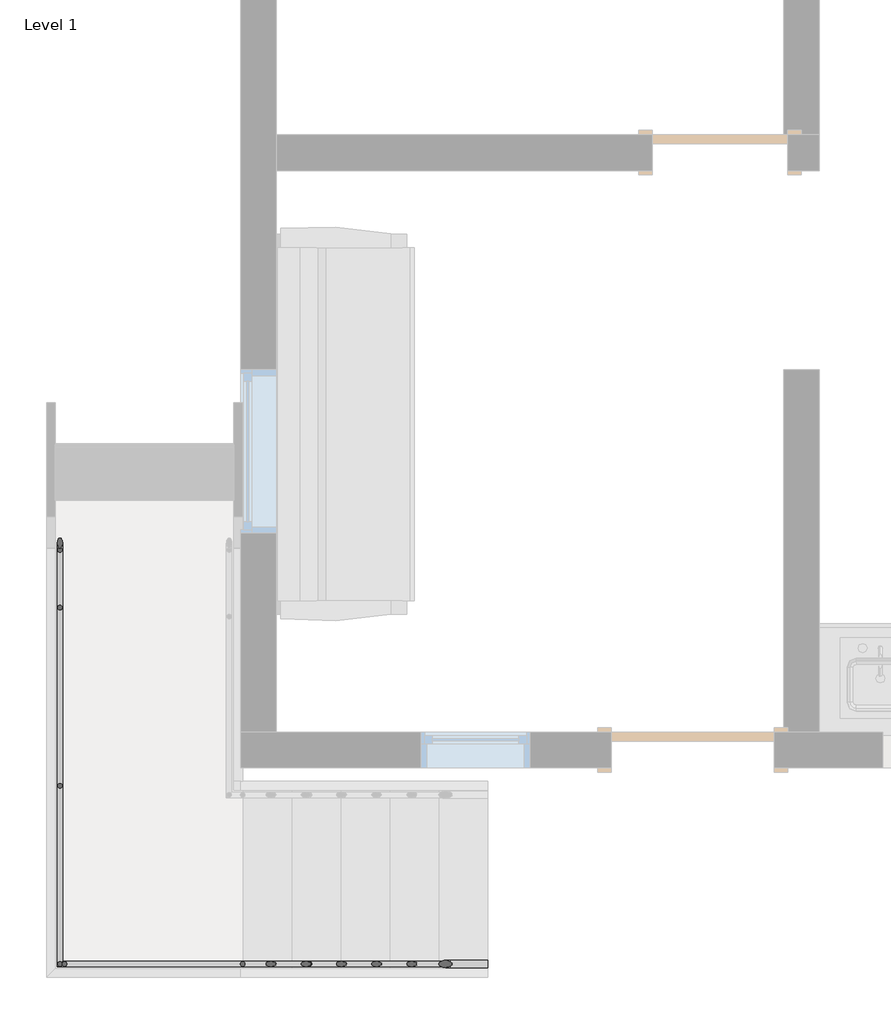
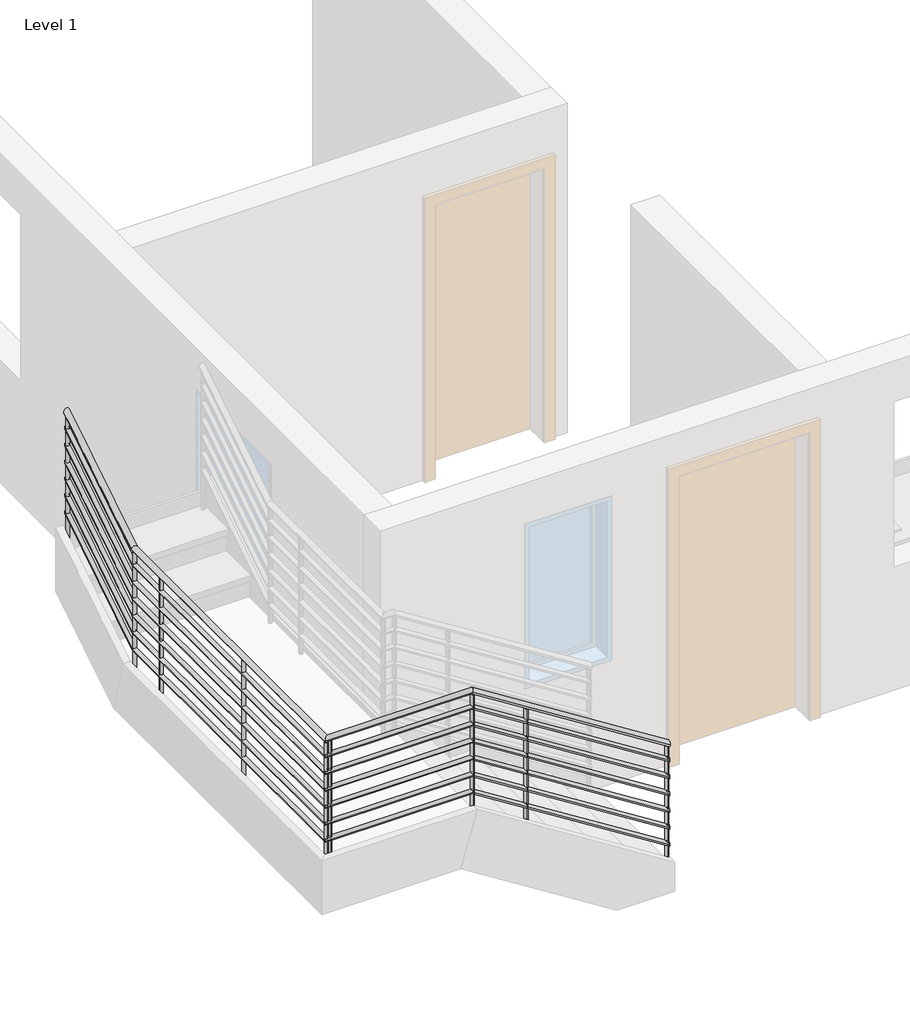
# One storey, part 2 of 3: 1 railing.
"""IFC4 building model written with IfcOpenShell, lengths in millimetres."""

from ifc_helpers import new_model, si_unit, point, frame, frame_2d, origin, place, context, project, spatial, circle_curve, ellipse_curve, trimmed, segment, composite_curve, outline, extrude, element, save
from ifc_brep_helpers import plane_surface, cylinder_surface, advanced_brep

model = new_model("IFC4")

# Units and contexts
model_context = context("Model", 3, world=origin())
ifc_project = project(units=[si_unit("LENGTHUNIT", "METRE", prefix="MILLI")], contexts=[model_context])

# Site, building, storey
site = spatial("IfcSite", under=ifc_project)
building = spatial("IfcBuilding", under=site)
storey = spatial("IfcBuildingStorey", under=building, Name="Level 1", Elevation=0.0)

# Railing
placement = place(None, origin())
element("IfcRailing", 1, ObjectType="900mm Pipe", at=placement, inside=storey, context=model_context, shape_type="SolidModel", body=[
    advanced_brep(
    [(-10176.2529994, 4755.2403022, 1050.2491997), (-10176.2529994, 4715.2403022, 1050.2491997), (-11557.0464524, 4755.2403022, 1923.4782609), (-11557.0464524, 4715.2403022, 1923.4782609), (-12556.6787807, 4755.2403022, 1923.4782609), (-12596.6787807, 4715.2403022, 1923.4782609), (-12556.6787807, 7064.6595365, 1923.4782609), (-12596.6787807, 7064.6595365, 1923.4782609), (-12556.6787807, 7883.8660835, 2441.5535475), (-12596.6787807, 7883.8660835, 2441.5535475)],
    [
        (0, 1, ellipse_curve(frame((-10176.2529994, 4735.2403022, 1050.2491997), z_axis=(1.0, 0.0, 0.0), x_axis=(0.0, 0.0, -1.0)), 23.6638438, 20.0)),
        (1, 0, ellipse_curve(frame((-10176.2529994, 4735.2403022, 1050.2491997), z_axis=(1.0, 0.0, 0.0), x_axis=(0.0, 0.0, -1.0)), 23.6638438, 20.0)),
        (0, 2),
        (2, 3, ellipse_curve(frame((-11557.0464524, 4735.2403022, 1923.4782609), z_axis=(0.9605132043335073, 0.0, -0.2782344053149754), x_axis=(-0.278234405314975, 0.0, -0.9605132043335074)), 20.822202, 20.0)),
        (3, 1),
        (3, 2, ellipse_curve(frame((-11557.0464524, 4735.2403022, 1923.4782609), z_axis=(0.9605132043335073, 0.0, -0.2782344053149754), x_axis=(-0.278234405314975, 0.0, -0.9605132043335074)), 20.822202, 20.0)),
        (2, 4),
        (4, 5, ellipse_curve(frame((-12576.6787807, 4735.2403022, 1923.4782609), z_axis=(0.7071067811865425, -0.7071067811865526, 0.0), x_axis=(0.7071067811865526, 0.7071067811865424, 0.0)), 28.2842712, 20.0)),
        (5, 3),
        (5, 4, ellipse_curve(frame((-12576.6787807, 4735.2403022, 1923.4782609), z_axis=(0.7071067811865425, -0.7071067811865526, 0.0), x_axis=(0.7071067811865526, 0.7071067811865424, 0.0)), 28.2842712, 20.0)),
        (4, 6),
        (6, 7, ellipse_curve(frame((-12576.6787807, 7064.6595365, 1923.4782609), z_axis=(0.0, -0.9605132043335083, -0.27823440531497184), x_axis=(0.0, -0.27823440531497223, 0.9605132043335083)), 20.822202, 20.0)),
        (7, 5),
        (7, 6, ellipse_curve(frame((-12576.6787807, 7064.6595365, 1923.4782609), z_axis=(0.0, -0.9605132043335083, -0.27823440531497184), x_axis=(0.0, -0.27823440531497223, 0.9605132043335083)), 20.822202, 20.0)),
        (8, 9, ellipse_curve(frame((-12576.6787807, 7883.8660835, 2441.5535475), z_axis=(0.0, 1.0, 0.0), x_axis=(0.0, 0.0, -1.0)), 23.6638438, 20.0)),
        (9, 8, ellipse_curve(frame((-12576.6787807, 7883.8660835, 2441.5535475), z_axis=(0.0, 1.0, 0.0), x_axis=(0.0, 0.0, -1.0)), 23.6638438, 20.0)),
        (6, 8),
        (9, 7),
    ],
    [
        plane_surface(frame((-10176.2529994, 4735.2403022, 1073.9130435), z_axis=(1.0, 0.0, 0.0), x_axis=(0.0, -1.0, 0.0))),
        cylinder_surface(frame((-10186.9429122, 4735.2403022, 1057.0096189), z_axis=(0.845171231398044, 0.0, -0.5344956404098298), x_axis=(0.0, -1.0, 0.0)), 20.0),
        cylinder_surface(frame((-11551.2529994, 4735.2403022, 1923.4782609), z_axis=(1.0, 0.0, 0.0), x_axis=(0.0, -1.0, 0.0)), 20.0),
        cylinder_surface(frame((-12576.6787807, 4735.2403022, 1923.4782609), z_axis=(0.0, -1.0, 0.0), x_axis=(-1.0, 0.0, 0.0)), 20.0),
        plane_surface(frame((-12576.6787807, 7883.8660835, 2465.2173913), z_axis=(0.0, 1.0, 0.0), x_axis=(0.0, 0.0, 1.0))),
        cylinder_surface(frame((-12576.6787807, 7069.5559963, 1926.5748362), z_axis=(0.0, -0.845171231398048, -0.5344956404098234), x_axis=(-1.0, 0.0, 0.0)), 20.0),
    ],
    [
        (0, [[1, 2]]),
        (1, [[-1, 3, 4, 5]]),
        (1, [[-2, -5, 6, -3]]),
        (2, [[-4, 7, 8, 9]]),
        (2, [[-6, -9, 10, -7]]),
        (3, [[-8, 11, 12, 13]]),
        (3, [[-10, -13, 14, -11]]),
        (4, [[15, 16]]),
        (5, [[-12, 17, -16, 18]]),
        (5, [[-14, -18, -15, -17]]),
    ],
),
    advanced_brep(
    [(-10176.2529994, 4750.2403022, 931.1651606), (-10176.2529994, 4720.2403022, 931.1651606), (-11555.5980892, 4750.2403022, 1803.4782609), (-11555.5980892, 4720.2403022, 1803.4782609), (-12561.6787807, 4750.2403022, 1803.4782609), (-12591.6787807, 4720.2403022, 1803.4782609), (-12561.6787807, 7063.2111733, 1803.4782609), (-12591.6787807, 7063.2111733, 1803.4782609), (-12561.6787807, 7883.8660835, 2322.4695085), (-12591.6787807, 7883.8660835, 2322.4695085)],
    [
        (0, 1, ellipse_curve(frame((-10176.2529994, 4735.2403022, 931.1651606), z_axis=(1.0, 0.0, 0.0), x_axis=(0.0, 0.0, -1.0)), 17.7478828, 15.0)),
        (1, 0, ellipse_curve(frame((-10176.2529994, 4735.2403022, 931.1651606), z_axis=(1.0, 0.0, 0.0), x_axis=(0.0, 0.0, -1.0)), 17.7478828, 15.0)),
        (0, 2),
        (2, 3, ellipse_curve(frame((-11555.5980892, 4735.2403022, 1803.4782609), z_axis=(0.9605132043335073, 0.0, -0.27823440531497534), x_axis=(-0.27823440531497506, 0.0, -0.9605132043335075)), 15.6166515, 15.0)),
        (3, 1),
        (3, 2, ellipse_curve(frame((-11555.5980892, 4735.2403022, 1803.4782609), z_axis=(0.9605132043335073, 0.0, -0.27823440531497534), x_axis=(-0.27823440531497506, 0.0, -0.9605132043335075)), 15.6166515, 15.0)),
        (2, 4),
        (4, 5, ellipse_curve(frame((-12576.6787807, 4735.2403022, 1803.4782609), z_axis=(0.7071067811865425, -0.7071067811865526, 0.0), x_axis=(0.7071067811865526, 0.7071067811865424, 0.0)), 21.2132034, 15.0)),
        (5, 3),
        (5, 4, ellipse_curve(frame((-12576.6787807, 4735.2403022, 1803.4782609), z_axis=(0.7071067811865425, -0.7071067811865526, 0.0), x_axis=(0.7071067811865526, 0.7071067811865424, 0.0)), 21.2132034, 15.0)),
        (4, 6),
        (6, 7, ellipse_curve(frame((-12576.6787807, 7063.2111733, 1803.4782609), z_axis=(0.0, -0.9605132043335083, -0.27823440531497196), x_axis=(0.0, -0.2782344053149721, 0.9605132043335084)), 15.6166515, 15.0)),
        (7, 5),
        (7, 6, ellipse_curve(frame((-12576.6787807, 7063.2111733, 1803.4782609), z_axis=(0.0, -0.9605132043335083, -0.27823440531497196), x_axis=(0.0, -0.2782344053149721, 0.9605132043335084)), 15.6166515, 15.0)),
        (8, 9, ellipse_curve(frame((-12576.6787807, 7883.8660835, 2322.4695085), z_axis=(0.0, 1.0, 0.0), x_axis=(0.0, 0.0, -1.0)), 17.7478828, 15.0)),
        (9, 8, ellipse_curve(frame((-12576.6787807, 7883.8660835, 2322.4695085), z_axis=(0.0, 1.0, 0.0), x_axis=(0.0, 0.0, -1.0)), 17.7478828, 15.0)),
        (6, 8),
        (9, 7),
    ],
    [
        plane_surface(frame((-10176.2529994, 4735.2403022, 948.9130435), z_axis=(1.0, 0.0, 0.0), x_axis=(0.0, -1.0, 0.0))),
        cylinder_surface(frame((-10184.270434, 4735.2403022, 936.235475), z_axis=(0.845171231398044, 0.0, -0.5344956404098297), x_axis=(0.0, -1.0, 0.0)), 15.0),
        cylinder_surface(frame((-11551.2529994, 4735.2403022, 1803.4782609), z_axis=(1.0, 0.0, 0.0), x_axis=(0.0, -1.0, 0.0)), 15.0),
        cylinder_surface(frame((-12576.6787807, 4735.2403022, 1803.4782609), z_axis=(0.0, -1.0, 0.0), x_axis=(-1.0, 0.0, 0.0)), 15.0),
        plane_surface(frame((-12576.6787807, 7883.8660835, 2340.2173913), z_axis=(0.0, 1.0, 0.0), x_axis=(0.0, 0.0, 1.0))),
        cylinder_surface(frame((-12576.6787807, 7066.8835181, 1805.8006924), z_axis=(0.0, -0.8451712313980478, -0.5344956404098237), x_axis=(-1.0, 0.0, 0.0)), 15.0),
    ],
    [
        (0, [[1, 2]]),
        (1, [[-1, 3, 4, 5]]),
        (1, [[-2, -5, 6, -3]]),
        (2, [[-4, 7, 8, 9]]),
        (2, [[-6, -9, 10, -7]]),
        (3, [[-8, 11, 12, 13]]),
        (3, [[-10, -13, 14, -11]]),
        (4, [[15, 16]]),
        (5, [[-12, 17, -16, 18]]),
        (5, [[-14, -18, -15, -17]]),
    ],
),
    advanced_brep(
    [(-10176.2529994, 4750.2403022, 806.1651606), (-10176.2529994, 4720.2403022, 806.1651606), (-11555.5980892, 4750.2403022, 1678.4782609), (-11555.5980892, 4720.2403022, 1678.4782609), (-12561.6787807, 4750.2403022, 1678.4782609), (-12591.6787807, 4720.2403022, 1678.4782609), (-12561.6787807, 7063.2111733, 1678.4782609), (-12591.6787807, 7063.2111733, 1678.4782609), (-12561.6787807, 7883.8660835, 2197.4695085), (-12591.6787807, 7883.8660835, 2197.4695085)],
    [
        (0, 1, ellipse_curve(frame((-10176.2529994, 4735.2403022, 806.1651606), z_axis=(1.0, 0.0, 0.0), x_axis=(0.0, 0.0, -1.0)), 17.7478828, 15.0)),
        (1, 0, ellipse_curve(frame((-10176.2529994, 4735.2403022, 806.1651606), z_axis=(1.0, 0.0, 0.0), x_axis=(0.0, 0.0, -1.0)), 17.7478828, 15.0)),
        (0, 2),
        (2, 3, ellipse_curve(frame((-11555.5980892, 4735.2403022, 1678.4782609), z_axis=(0.9605132043335073, 0.0, -0.27823440531497534), x_axis=(-0.27823440531497506, 0.0, -0.9605132043335075)), 15.6166515, 15.0)),
        (3, 1),
        (3, 2, ellipse_curve(frame((-11555.5980892, 4735.2403022, 1678.4782609), z_axis=(0.9605132043335073, 0.0, -0.27823440531497534), x_axis=(-0.27823440531497506, 0.0, -0.9605132043335075)), 15.6166515, 15.0)),
        (2, 4),
        (4, 5, ellipse_curve(frame((-12576.6787807, 4735.2403022, 1678.4782609), z_axis=(0.7071067811865425, -0.7071067811865526, 0.0), x_axis=(0.7071067811865526, 0.7071067811865424, 0.0)), 21.2132034, 15.0)),
        (5, 3),
        (5, 4, ellipse_curve(frame((-12576.6787807, 4735.2403022, 1678.4782609), z_axis=(0.7071067811865425, -0.7071067811865526, 0.0), x_axis=(0.7071067811865526, 0.7071067811865424, 0.0)), 21.2132034, 15.0)),
        (4, 6),
        (6, 7, ellipse_curve(frame((-12576.6787807, 7063.2111733, 1678.4782609), z_axis=(0.0, -0.9605132043335083, -0.27823440531497196), x_axis=(0.0, -0.2782344053149721, 0.9605132043335084)), 15.6166515, 15.0)),
        (7, 5),
        (7, 6, ellipse_curve(frame((-12576.6787807, 7063.2111733, 1678.4782609), z_axis=(0.0, -0.9605132043335083, -0.27823440531497196), x_axis=(0.0, -0.2782344053149721, 0.9605132043335084)), 15.6166515, 15.0)),
        (8, 9, ellipse_curve(frame((-12576.6787807, 7883.8660835, 2197.4695085), z_axis=(0.0, 1.0, 0.0), x_axis=(0.0, 0.0, -1.0)), 17.7478828, 15.0)),
        (9, 8, ellipse_curve(frame((-12576.6787807, 7883.8660835, 2197.4695085), z_axis=(0.0, 1.0, 0.0), x_axis=(0.0, 0.0, -1.0)), 17.7478828, 15.0)),
        (6, 8),
        (9, 7),
    ],
    [
        plane_surface(frame((-10176.2529994, 4735.2403022, 823.9130435), z_axis=(1.0, 0.0, 0.0), x_axis=(0.0, -1.0, 0.0))),
        cylinder_surface(frame((-10184.270434, 4735.2403022, 811.235475), z_axis=(0.845171231398044, 0.0, -0.5344956404098297), x_axis=(0.0, -1.0, 0.0)), 15.0),
        cylinder_surface(frame((-11551.2529994, 4735.2403022, 1678.4782609), z_axis=(1.0, 0.0, 0.0), x_axis=(0.0, -1.0, 0.0)), 15.0),
        cylinder_surface(frame((-12576.6787807, 4735.2403022, 1678.4782609), z_axis=(0.0, -1.0, 0.0), x_axis=(-1.0, 0.0, 0.0)), 15.0),
        plane_surface(frame((-12576.6787807, 7883.8660835, 2215.2173913), z_axis=(0.0, 1.0, 0.0), x_axis=(0.0, 0.0, 1.0))),
        cylinder_surface(frame((-12576.6787807, 7066.8835181, 1680.8006924), z_axis=(0.0, -0.8451712313980478, -0.5344956404098237), x_axis=(-1.0, 0.0, 0.0)), 15.0),
    ],
    [
        (0, [[1, 2]]),
        (1, [[-1, 3, 4, 5]]),
        (1, [[-2, -5, 6, -3]]),
        (2, [[-4, 7, 8, 9]]),
        (2, [[-6, -9, 10, -7]]),
        (3, [[-8, 11, 12, 13]]),
        (3, [[-10, -13, 14, -11]]),
        (4, [[15, 16]]),
        (5, [[-12, 17, -16, 18]]),
        (5, [[-14, -18, -15, -17]]),
    ],
),
    advanced_brep(
    [(-10176.2529994, 4750.2403022, 681.1651606), (-10176.2529994, 4720.2403022, 681.1651606), (-11555.5980892, 4750.2403022, 1553.4782609), (-11555.5980892, 4720.2403022, 1553.4782609), (-12561.6787807, 4750.2403022, 1553.4782609), (-12591.6787807, 4720.2403022, 1553.4782609), (-12561.6787807, 7063.2111733, 1553.4782609), (-12591.6787807, 7063.2111733, 1553.4782609), (-12561.6787807, 7883.8660835, 2072.4695085), (-12591.6787807, 7883.8660835, 2072.4695085)],
    [
        (0, 1, ellipse_curve(frame((-10176.2529994, 4735.2403022, 681.1651606), z_axis=(1.0, 0.0, 0.0), x_axis=(0.0, 0.0, -1.0)), 17.7478828, 15.0)),
        (1, 0, ellipse_curve(frame((-10176.2529994, 4735.2403022, 681.1651606), z_axis=(1.0, 0.0, 0.0), x_axis=(0.0, 0.0, -1.0)), 17.7478828, 15.0)),
        (0, 2),
        (2, 3, ellipse_curve(frame((-11555.5980892, 4735.2403022, 1553.4782609), z_axis=(0.9605132043335073, 0.0, -0.27823440531497534), x_axis=(-0.27823440531497506, 0.0, -0.9605132043335075)), 15.6166515, 15.0)),
        (3, 1),
        (3, 2, ellipse_curve(frame((-11555.5980892, 4735.2403022, 1553.4782609), z_axis=(0.9605132043335073, 0.0, -0.27823440531497534), x_axis=(-0.27823440531497506, 0.0, -0.9605132043335075)), 15.6166515, 15.0)),
        (2, 4),
        (4, 5, ellipse_curve(frame((-12576.6787807, 4735.2403022, 1553.4782609), z_axis=(0.7071067811865425, -0.7071067811865526, 0.0), x_axis=(0.7071067811865526, 0.7071067811865424, 0.0)), 21.2132034, 15.0)),
        (5, 3),
        (5, 4, ellipse_curve(frame((-12576.6787807, 4735.2403022, 1553.4782609), z_axis=(0.7071067811865425, -0.7071067811865526, 0.0), x_axis=(0.7071067811865526, 0.7071067811865424, 0.0)), 21.2132034, 15.0)),
        (4, 6),
        (6, 7, ellipse_curve(frame((-12576.6787807, 7063.2111733, 1553.4782609), z_axis=(0.0, -0.9605132043335083, -0.27823440531497196), x_axis=(0.0, -0.2782344053149721, 0.9605132043335084)), 15.6166515, 15.0)),
        (7, 5),
        (7, 6, ellipse_curve(frame((-12576.6787807, 7063.2111733, 1553.4782609), z_axis=(0.0, -0.9605132043335083, -0.27823440531497196), x_axis=(0.0, -0.2782344053149721, 0.9605132043335084)), 15.6166515, 15.0)),
        (8, 9, ellipse_curve(frame((-12576.6787807, 7883.8660835, 2072.4695085), z_axis=(0.0, 1.0, 0.0), x_axis=(0.0, 0.0, -1.0)), 17.7478828, 15.0)),
        (9, 8, ellipse_curve(frame((-12576.6787807, 7883.8660835, 2072.4695085), z_axis=(0.0, 1.0, 0.0), x_axis=(0.0, 0.0, -1.0)), 17.7478828, 15.0)),
        (6, 8),
        (9, 7),
    ],
    [
        plane_surface(frame((-10176.2529994, 4735.2403022, 698.9130435), z_axis=(1.0, 0.0, 0.0), x_axis=(0.0, -1.0, 0.0))),
        cylinder_surface(frame((-10184.270434, 4735.2403022, 686.235475), z_axis=(0.845171231398044, 0.0, -0.5344956404098297), x_axis=(0.0, -1.0, 0.0)), 15.0),
        cylinder_surface(frame((-11551.2529994, 4735.2403022, 1553.4782609), z_axis=(1.0, 0.0, 0.0), x_axis=(0.0, -1.0, 0.0)), 15.0),
        cylinder_surface(frame((-12576.6787807, 4735.2403022, 1553.4782609), z_axis=(0.0, -1.0, 0.0), x_axis=(-1.0, 0.0, 0.0)), 15.0),
        plane_surface(frame((-12576.6787807, 7883.8660835, 2090.2173913), z_axis=(0.0, 1.0, 0.0), x_axis=(0.0, 0.0, 1.0))),
        cylinder_surface(frame((-12576.6787807, 7066.8835181, 1555.8006924), z_axis=(0.0, -0.8451712313980478, -0.5344956404098237), x_axis=(-1.0, 0.0, 0.0)), 15.0),
    ],
    [
        (0, [[1, 2]]),
        (1, [[-1, 3, 4, 5]]),
        (1, [[-2, -5, 6, -3]]),
        (2, [[-4, 7, 8, 9]]),
        (2, [[-6, -9, 10, -7]]),
        (3, [[-8, 11, 12, 13]]),
        (3, [[-10, -13, 14, -11]]),
        (4, [[15, 16]]),
        (5, [[-12, 17, -16, 18]]),
        (5, [[-14, -18, -15, -17]]),
    ],
),
    advanced_brep(
    [(-10176.2529994, 4750.2403022, 556.1651606), (-10176.2529994, 4720.2403022, 556.1651606), (-11555.5980892, 4750.2403022, 1428.4782609), (-11555.5980892, 4720.2403022, 1428.4782609), (-12561.6787807, 4750.2403022, 1428.4782609), (-12591.6787807, 4720.2403022, 1428.4782609), (-12561.6787807, 7063.2111733, 1428.4782609), (-12591.6787807, 7063.2111733, 1428.4782609), (-12561.6787807, 7883.8660835, 1947.4695085), (-12591.6787807, 7883.8660835, 1947.4695085)],
    [
        (0, 1, ellipse_curve(frame((-10176.2529994, 4735.2403022, 556.1651606), z_axis=(1.0, 0.0, 0.0), x_axis=(0.0, 0.0, -1.0)), 17.7478828, 15.0)),
        (1, 0, ellipse_curve(frame((-10176.2529994, 4735.2403022, 556.1651606), z_axis=(1.0, 0.0, 0.0), x_axis=(0.0, 0.0, -1.0)), 17.7478828, 15.0)),
        (0, 2),
        (2, 3, ellipse_curve(frame((-11555.5980892, 4735.2403022, 1428.4782609), z_axis=(0.9605132043335073, 0.0, -0.27823440531497534), x_axis=(-0.27823440531497506, 0.0, -0.9605132043335075)), 15.6166515, 15.0)),
        (3, 1),
        (3, 2, ellipse_curve(frame((-11555.5980892, 4735.2403022, 1428.4782609), z_axis=(0.9605132043335073, 0.0, -0.27823440531497534), x_axis=(-0.27823440531497506, 0.0, -0.9605132043335075)), 15.6166515, 15.0)),
        (2, 4),
        (4, 5, ellipse_curve(frame((-12576.6787807, 4735.2403022, 1428.4782609), z_axis=(0.7071067811865425, -0.7071067811865526, 0.0), x_axis=(0.7071067811865526, 0.7071067811865424, 0.0)), 21.2132034, 15.0)),
        (5, 3),
        (5, 4, ellipse_curve(frame((-12576.6787807, 4735.2403022, 1428.4782609), z_axis=(0.7071067811865425, -0.7071067811865526, 0.0), x_axis=(0.7071067811865526, 0.7071067811865424, 0.0)), 21.2132034, 15.0)),
        (4, 6),
        (6, 7, ellipse_curve(frame((-12576.6787807, 7063.2111733, 1428.4782609), z_axis=(0.0, -0.9605132043335083, -0.27823440531497196), x_axis=(0.0, -0.2782344053149721, 0.9605132043335084)), 15.6166515, 15.0)),
        (7, 5),
        (7, 6, ellipse_curve(frame((-12576.6787807, 7063.2111733, 1428.4782609), z_axis=(0.0, -0.9605132043335083, -0.27823440531497196), x_axis=(0.0, -0.2782344053149721, 0.9605132043335084)), 15.6166515, 15.0)),
        (8, 9, ellipse_curve(frame((-12576.6787807, 7883.8660835, 1947.4695085), z_axis=(0.0, 1.0, 0.0), x_axis=(0.0, 0.0, -1.0)), 17.7478828, 15.0)),
        (9, 8, ellipse_curve(frame((-12576.6787807, 7883.8660835, 1947.4695085), z_axis=(0.0, 1.0, 0.0), x_axis=(0.0, 0.0, -1.0)), 17.7478828, 15.0)),
        (6, 8),
        (9, 7),
    ],
    [
        plane_surface(frame((-10176.2529994, 4735.2403022, 573.9130435), z_axis=(1.0, 0.0, 0.0), x_axis=(0.0, -1.0, 0.0))),
        cylinder_surface(frame((-10184.270434, 4735.2403022, 561.235475), z_axis=(0.845171231398044, 0.0, -0.5344956404098297), x_axis=(0.0, -1.0, 0.0)), 15.0),
        cylinder_surface(frame((-11551.2529994, 4735.2403022, 1428.4782609), z_axis=(1.0, 0.0, 0.0), x_axis=(0.0, -1.0, 0.0)), 15.0),
        cylinder_surface(frame((-12576.6787807, 4735.2403022, 1428.4782609), z_axis=(0.0, -1.0, 0.0), x_axis=(-1.0, 0.0, 0.0)), 15.0),
        plane_surface(frame((-12576.6787807, 7883.8660835, 1965.2173913), z_axis=(0.0, 1.0, 0.0), x_axis=(0.0, 0.0, 1.0))),
        cylinder_surface(frame((-12576.6787807, 7066.8835181, 1430.8006924), z_axis=(0.0, -0.8451712313980478, -0.5344956404098237), x_axis=(-1.0, 0.0, 0.0)), 15.0),
    ],
    [
        (0, [[1, 2]]),
        (1, [[-1, 3, 4, 5]]),
        (1, [[-2, -5, 6, -3]]),
        (2, [[-4, 7, 8, 9]]),
        (2, [[-6, -9, 10, -7]]),
        (3, [[-8, 11, 12, 13]]),
        (3, [[-10, -13, 14, -11]]),
        (4, [[15, 16]]),
        (5, [[-12, 17, -16, 18]]),
        (5, [[-14, -18, -15, -17]]),
    ],
),
    advanced_brep(
    [(-10176.2529994, 4750.2403022, 431.1651606), (-10176.2529994, 4720.2403022, 431.1651606), (-11555.5980892, 4750.2403022, 1303.4782609), (-11555.5980892, 4720.2403022, 1303.4782609), (-12561.6787807, 4750.2403022, 1303.4782609), (-12591.6787807, 4720.2403022, 1303.4782609), (-12561.6787807, 7063.2111733, 1303.4782609), (-12591.6787807, 7063.2111733, 1303.4782609), (-12561.6787807, 7883.8660835, 1822.4695085), (-12591.6787807, 7883.8660835, 1822.4695085)],
    [
        (0, 1, ellipse_curve(frame((-10176.2529994, 4735.2403022, 431.1651606), z_axis=(1.0, 0.0, 0.0), x_axis=(0.0, 0.0, -1.0)), 17.7478828, 15.0)),
        (1, 0, ellipse_curve(frame((-10176.2529994, 4735.2403022, 431.1651606), z_axis=(1.0, 0.0, 0.0), x_axis=(0.0, 0.0, -1.0)), 17.7478828, 15.0)),
        (0, 2),
        (2, 3, ellipse_curve(frame((-11555.5980892, 4735.2403022, 1303.4782609), z_axis=(0.9605132043335073, 0.0, -0.27823440531497534), x_axis=(-0.27823440531497506, 0.0, -0.9605132043335075)), 15.6166515, 15.0)),
        (3, 1),
        (3, 2, ellipse_curve(frame((-11555.5980892, 4735.2403022, 1303.4782609), z_axis=(0.9605132043335073, 0.0, -0.27823440531497534), x_axis=(-0.27823440531497506, 0.0, -0.9605132043335075)), 15.6166515, 15.0)),
        (2, 4),
        (4, 5, ellipse_curve(frame((-12576.6787807, 4735.2403022, 1303.4782609), z_axis=(0.7071067811865425, -0.7071067811865526, 0.0), x_axis=(0.7071067811865526, 0.7071067811865424, 0.0)), 21.2132034, 15.0)),
        (5, 3),
        (5, 4, ellipse_curve(frame((-12576.6787807, 4735.2403022, 1303.4782609), z_axis=(0.7071067811865425, -0.7071067811865526, 0.0), x_axis=(0.7071067811865526, 0.7071067811865424, 0.0)), 21.2132034, 15.0)),
        (4, 6),
        (6, 7, ellipse_curve(frame((-12576.6787807, 7063.2111733, 1303.4782609), z_axis=(0.0, -0.9605132043335083, -0.27823440531497196), x_axis=(0.0, -0.2782344053149721, 0.9605132043335084)), 15.6166515, 15.0)),
        (7, 5),
        (7, 6, ellipse_curve(frame((-12576.6787807, 7063.2111733, 1303.4782609), z_axis=(0.0, -0.9605132043335083, -0.27823440531497196), x_axis=(0.0, -0.2782344053149721, 0.9605132043335084)), 15.6166515, 15.0)),
        (8, 9, ellipse_curve(frame((-12576.6787807, 7883.8660835, 1822.4695085), z_axis=(0.0, 1.0, 0.0), x_axis=(0.0, 0.0, -1.0)), 17.7478828, 15.0)),
        (9, 8, ellipse_curve(frame((-12576.6787807, 7883.8660835, 1822.4695085), z_axis=(0.0, 1.0, 0.0), x_axis=(0.0, 0.0, -1.0)), 17.7478828, 15.0)),
        (6, 8),
        (9, 7),
    ],
    [
        plane_surface(frame((-10176.2529994, 4735.2403022, 448.9130435), z_axis=(1.0, 0.0, 0.0), x_axis=(0.0, -1.0, 0.0))),
        cylinder_surface(frame((-10184.270434, 4735.2403022, 436.235475), z_axis=(0.845171231398044, 0.0, -0.5344956404098297), x_axis=(0.0, -1.0, 0.0)), 15.0),
        cylinder_surface(frame((-11551.2529994, 4735.2403022, 1303.4782609), z_axis=(1.0, 0.0, 0.0), x_axis=(0.0, -1.0, 0.0)), 15.0),
        cylinder_surface(frame((-12576.6787807, 4735.2403022, 1303.4782609), z_axis=(0.0, -1.0, 0.0), x_axis=(-1.0, 0.0, 0.0)), 15.0),
        plane_surface(frame((-12576.6787807, 7883.8660835, 1840.2173913), z_axis=(0.0, 1.0, 0.0), x_axis=(0.0, 0.0, 1.0))),
        cylinder_surface(frame((-12576.6787807, 7066.8835181, 1305.8006924), z_axis=(0.0, -0.8451712313980478, -0.5344956404098237), x_axis=(-1.0, 0.0, 0.0)), 15.0),
    ],
    [
        (0, [[1, 2]]),
        (1, [[-1, 3, 4, 5]]),
        (1, [[-2, -5, 6, -3]]),
        (2, [[-4, 7, 8, 9]]),
        (2, [[-6, -9, 10, -7]]),
        (3, [[-8, 11, 12, 13]]),
        (3, [[-10, -13, 14, -11]]),
        (4, [[15, 16]]),
        (5, [[-12, 17, -16, 18]]),
        (5, [[-14, -18, -15, -17]]),
    ],
),
    advanced_brep(
    [(-10176.2529994, 4750.2403022, 306.1651606), (-10176.2529994, 4720.2403022, 306.1651606), (-11555.5980892, 4750.2403022, 1178.4782609), (-11555.5980892, 4720.2403022, 1178.4782609), (-12561.6787807, 4750.2403022, 1178.4782609), (-12591.6787807, 4720.2403022, 1178.4782609), (-12561.6787807, 7063.2111733, 1178.4782609), (-12591.6787807, 7063.2111733, 1178.4782609), (-12561.6787807, 7883.8660835, 1697.4695085), (-12591.6787807, 7883.8660835, 1697.4695085)],
    [
        (0, 1, ellipse_curve(frame((-10176.2529994, 4735.2403022, 306.1651606), z_axis=(1.0, 0.0, 0.0), x_axis=(0.0, 0.0, -1.0)), 17.7478828, 15.0)),
        (1, 0, ellipse_curve(frame((-10176.2529994, 4735.2403022, 306.1651606), z_axis=(1.0, 0.0, 0.0), x_axis=(0.0, 0.0, -1.0)), 17.7478828, 15.0)),
        (0, 2),
        (2, 3, ellipse_curve(frame((-11555.5980892, 4735.2403022, 1178.4782609), z_axis=(0.9605132043335073, 0.0, -0.27823440531497534), x_axis=(-0.27823440531497506, 0.0, -0.9605132043335075)), 15.6166515, 15.0)),
        (3, 1),
        (3, 2, ellipse_curve(frame((-11555.5980892, 4735.2403022, 1178.4782609), z_axis=(0.9605132043335073, 0.0, -0.27823440531497534), x_axis=(-0.27823440531497506, 0.0, -0.9605132043335075)), 15.6166515, 15.0)),
        (2, 4),
        (4, 5, ellipse_curve(frame((-12576.6787807, 4735.2403022, 1178.4782609), z_axis=(0.7071067811865425, -0.7071067811865526, 0.0), x_axis=(0.7071067811865526, 0.7071067811865424, 0.0)), 21.2132034, 15.0)),
        (5, 3),
        (5, 4, ellipse_curve(frame((-12576.6787807, 4735.2403022, 1178.4782609), z_axis=(0.7071067811865425, -0.7071067811865526, 0.0), x_axis=(0.7071067811865526, 0.7071067811865424, 0.0)), 21.2132034, 15.0)),
        (4, 6),
        (6, 7, ellipse_curve(frame((-12576.6787807, 7063.2111733, 1178.4782609), z_axis=(0.0, -0.9605132043335083, -0.27823440531497196), x_axis=(0.0, -0.2782344053149721, 0.9605132043335084)), 15.6166515, 15.0)),
        (7, 5),
        (7, 6, ellipse_curve(frame((-12576.6787807, 7063.2111733, 1178.4782609), z_axis=(0.0, -0.9605132043335083, -0.27823440531497196), x_axis=(0.0, -0.2782344053149721, 0.9605132043335084)), 15.6166515, 15.0)),
        (8, 9, ellipse_curve(frame((-12576.6787807, 7883.8660835, 1697.4695085), z_axis=(0.0, 1.0, 0.0), x_axis=(0.0, 0.0, -1.0)), 17.7478828, 15.0)),
        (9, 8, ellipse_curve(frame((-12576.6787807, 7883.8660835, 1697.4695085), z_axis=(0.0, 1.0, 0.0), x_axis=(0.0, 0.0, -1.0)), 17.7478828, 15.0)),
        (6, 8),
        (9, 7),
    ],
    [
        plane_surface(frame((-10176.2529994, 4735.2403022, 323.9130435), z_axis=(1.0, 0.0, 0.0), x_axis=(0.0, -1.0, 0.0))),
        cylinder_surface(frame((-10184.270434, 4735.2403022, 311.235475), z_axis=(0.845171231398044, 0.0, -0.5344956404098297), x_axis=(0.0, -1.0, 0.0)), 15.0),
        cylinder_surface(frame((-11551.2529994, 4735.2403022, 1178.4782609), z_axis=(1.0, 0.0, 0.0), x_axis=(0.0, -1.0, 0.0)), 15.0),
        cylinder_surface(frame((-12576.6787807, 4735.2403022, 1178.4782609), z_axis=(0.0, -1.0, 0.0), x_axis=(-1.0, 0.0, 0.0)), 15.0),
        plane_surface(frame((-12576.6787807, 7883.8660835, 1715.2173913), z_axis=(0.0, 1.0, 0.0), x_axis=(0.0, 0.0, 1.0))),
        cylinder_surface(frame((-12576.6787807, 7066.8835181, 1180.8006924), z_axis=(0.0, -0.8451712313980478, -0.5344956404098237), x_axis=(-1.0, 0.0, 0.0)), 15.0),
    ],
    [
        (0, [[1, 2]]),
        (1, [[-1, 3, 4, 5]]),
        (1, [[-2, -5, 6, -3]]),
        (2, [[-4, 7, 8, 9]]),
        (2, [[-6, -9, 10, -7]]),
        (3, [[-8, 11, 12, 13]]),
        (3, [[-10, -13, 14, -11]]),
        (4, [[15, 16]]),
        (5, [[-12, 17, -16, 18]]),
        (5, [[-14, -18, -15, -17]]),
    ],
),
    extrude(outline(composite_curve([segment(trimmed(circle_curve(frame_2d((-12576.6787807, 6735.2403022)), 12.5), [point((-12564.1787807, 6735.2403022))], [point((-12589.1787807, 6735.2403022))], False, "CARTESIAN"), True, "CONTINUOUS"), segment(trimmed(circle_curve(frame_2d((-12576.6787807, 6735.2403022)), 12.5), [point((-12589.1787807, 6735.2403022))], [point((-12564.1787807, 6735.2403022))], False, "CARTESIAN"), True, "CONTINUOUS")], self_intersect=False)), frame((0.0, 0.0, 1043.4782609), z_axis=(0.0, 0.0, 1.0), x_axis=(1.0, 0.0, 0.0)), (0.0, 0.0, 1.0), 860.0),
    extrude(outline(composite_curve([segment(trimmed(circle_curve(frame_2d((-12576.6787807, 5735.2403022)), 12.5), [point((-12564.1787807, 5735.2403022))], [point((-12589.1787807, 5735.2403022))], False, "CARTESIAN"), True, "CONTINUOUS"), segment(trimmed(circle_curve(frame_2d((-12576.6787807, 5735.2403022)), 12.5), [point((-12589.1787807, 5735.2403022))], [point((-12564.1787807, 5735.2403022))], False, "CARTESIAN"), True, "CONTINUOUS")], self_intersect=False)), frame((0.0, 0.0, 1043.4782609), z_axis=(0.0, 0.0, 1.0), x_axis=(1.0, 0.0, 0.0)), (0.0, 0.0, 1.0), 860.0),
    extrude(outline(composite_curve([segment(trimmed(circle_curve(frame_2d((-12551.2529994, 4735.2403022)), 12.5), [point((-12551.2529994, 4747.7403022))], [point((-12551.2529994, 4722.7403022))], False, "CARTESIAN"), True, "CONTINUOUS"), segment(trimmed(circle_curve(frame_2d((-12551.2529994, 4735.2403022)), 12.5), [point((-12551.2529994, 4722.7403022))], [point((-12551.2529994, 4747.7403022))], False, "CARTESIAN"), True, "CONTINUOUS")], self_intersect=False)), frame((0.0, 0.0, 1043.4782609), z_axis=(0.0, 0.0, 1.0), x_axis=(1.0, 0.0, 0.0)), (0.0, 0.0, 1.0), 860.0),
    advanced_brep(
    [(-11176.2529994, 4722.7403022, 1658.9964231), (-11176.2529994, 4747.7403022, 1658.9964231), (-11176.2529994, 4747.7403022, 695.6521739), (-11176.2529994, 4722.7403022, 695.6521739)],
    [
        (0, 1, ellipse_curve(frame((-11176.2529994, 4735.2403022, 1658.9964231), z_axis=(-0.5344956404098302, 0.0, -0.8451712313980437), x_axis=(-0.8451712313980437, 0.0, 0.53449564040983)), 14.7899024, 12.5)),
        (1, 2),
        (2, 3, circle_curve(frame((-11176.2529994, 4735.2403022, 695.6521739), z_axis=(0.0, 0.0, 1.0), x_axis=(0.0, 1.0, 0.0)), 12.5)),
        (3, 0),
        (3, 2, circle_curve(frame((-11176.2529994, 4735.2403022, 695.6521739), z_axis=(0.0, 0.0, 1.0), x_axis=(0.0, 1.0, 0.0)), 12.5)),
        (1, 0, ellipse_curve(frame((-11176.2529994, 4735.2403022, 1658.9964231), z_axis=(-0.5344956404098302, 0.0, -0.8451712313980437), x_axis=(-0.8451712313980437, 0.0, 0.53449564040983)), 14.7899024, 12.5)),
    ],
    [
        cylinder_surface(frame((-11176.2529994, 4735.2403022, 595.6521739), z_axis=(0.0, 0.0, 1.0), x_axis=(0.0, 1.0, 0.0)), 12.5),
        plane_surface(frame((-11201.2529994, 4760.2403022, 1674.8066998), z_axis=(0.5344956404098302, 0.0, 0.8451712313980437), x_axis=(0.0, -1.0, 0.0))),
        plane_surface(frame((-11151.2529994, 4760.2403022, 695.6521739), z_axis=(0.0, 0.0, -1.0), x_axis=(0.0, -1.0, 0.0))),
    ],
    [
        (0, [[1, 2, 3, 4]]),
        (0, [[5, -2, 6, -4]]),
        (1, [[-6, -1]]),
        (2, [[-5, -3]]),
    ],
),
    extrude(outline(composite_curve([segment(trimmed(circle_curve(frame_2d((-12576.6787807, 7058.8660835)), 12.5), [point((-12564.1787807, 7058.8660835))], [point((-12589.1787807, 7058.8660835))], False, "CARTESIAN"), True, "CONTINUOUS"), segment(trimmed(circle_curve(frame_2d((-12576.6787807, 7058.8660835)), 12.5), [point((-12589.1787807, 7058.8660835))], [point((-12564.1787807, 7058.8660835))], False, "CARTESIAN"), True, "CONTINUOUS")], self_intersect=False)), frame((0.0, 0.0, 1043.4782609), z_axis=(0.0, 0.0, 1.0), x_axis=(1.0, 0.0, 0.0)), (0.0, 0.0, 1.0), 860.0),
    extrude(outline(composite_curve([segment(trimmed(circle_curve(frame_2d((-12576.6787807, 4735.2403022)), 12.5), [point((-12576.6787807, 4747.7403022))], [point((-12576.6787807, 4722.7403022))], False, "CARTESIAN"), True, "CONTINUOUS"), segment(trimmed(circle_curve(frame_2d((-12576.6787807, 4735.2403022)), 12.5), [point((-12576.6787807, 4722.7403022))], [point((-12576.6787807, 4747.7403022))], False, "CARTESIAN"), True, "CONTINUOUS")], self_intersect=False)), frame((0.0, 0.0, 1043.4782609), z_axis=(0.0, 0.0, 1.0), x_axis=(1.0, 0.0, 0.0)), (0.0, 0.0, 1.0), 860.0),
    advanced_brep(
    [(-11551.2529994, 4722.7403022, 1896.1505733), (-11551.2529994, 4747.7403022, 1896.1505733), (-11551.2529994, 4747.7403022, 1043.4782609), (-11551.2529994, 4722.7403022, 1043.4782609)],
    [
        (0, 1, ellipse_curve(frame((-11551.2529994, 4735.2403022, 1896.1505733), z_axis=(-0.5344956404098351, 0.0, -0.8451712313980406), x_axis=(-0.8451712313980405, 0.0, 0.5344956404098349)), 14.7899024, 12.5)),
        (1, 2),
        (2, 3, circle_curve(frame((-11551.2529994, 4735.2403022, 1043.4782609), z_axis=(0.0, 0.0, 1.0), x_axis=(0.0, 1.0, 0.0)), 12.5)),
        (3, 0),
        (3, 2, circle_curve(frame((-11551.2529994, 4735.2403022, 1043.4782609), z_axis=(0.0, 0.0, 1.0), x_axis=(0.0, 1.0, 0.0)), 12.5)),
        (1, 0, ellipse_curve(frame((-11551.2529994, 4735.2403022, 1896.1505733), z_axis=(-0.5344956404098351, 0.0, -0.8451712313980406), x_axis=(-0.8451712313980405, 0.0, 0.5344956404098349)), 14.7899024, 12.5)),
    ],
    [
        cylinder_surface(frame((-11551.2529994, 4735.2403022, 943.4782609), z_axis=(0.0, 0.0, 1.0), x_axis=(0.0, 1.0, 0.0)), 12.5),
        plane_surface(frame((-11576.2529994, 4760.2403022, 1911.96085), z_axis=(0.5344956404098351, 0.0, 0.8451712313980406), x_axis=(0.0, -1.0, 0.0))),
        plane_surface(frame((-11526.2529994, 4760.2403022, 1043.4782609), z_axis=(0.0, 0.0, -1.0), x_axis=(0.0, -1.0, 0.0))),
    ],
    [
        (0, [[1, 2, 3, 4]]),
        (0, [[5, -2, 6, -4]]),
        (1, [[-6, -1]]),
        (2, [[-5, -3]]),
    ],
),
    advanced_brep(
    [(-12589.1787807, 7871.3660835, 2409.9845654), (-12564.1787807, 7871.3660835, 2409.9845654), (-12564.1787807, 7871.3660835, 1391.3043478), (-12589.1787807, 7871.3660835, 1391.3043478)],
    [
        (0, 1, ellipse_curve(frame((-12576.6787807, 7871.3660835, 2409.9845654), z_axis=(0.0, 0.5344956404098351, -0.8451712313980406), x_axis=(0.0, 0.8451712313980405, 0.5344956404098349)), 14.7899024, 12.5)),
        (1, 2),
        (2, 3, circle_curve(frame((-12576.6787807, 7871.3660835, 1391.3043478), z_axis=(0.0, 0.0, 1.0), x_axis=(1.0, 0.0, 0.0)), 12.5)),
        (3, 0),
        (3, 2, circle_curve(frame((-12576.6787807, 7871.3660835, 1391.3043478), z_axis=(0.0, 0.0, 1.0), x_axis=(1.0, 0.0, 0.0)), 12.5)),
        (1, 0, ellipse_curve(frame((-12576.6787807, 7871.3660835, 2409.9845654), z_axis=(0.0, 0.5344956404098351, -0.8451712313980406), x_axis=(0.0, 0.8451712313980405, 0.5344956404098349)), 14.7899024, 12.5)),
    ],
    [
        cylinder_surface(frame((-12576.6787807, 7871.3660835, 1291.3043478), z_axis=(0.0, 0.0, 1.0), x_axis=(1.0, 0.0, 0.0)), 12.5),
        plane_surface(frame((-12551.6787807, 7896.3660835, 2425.7948421), z_axis=(0.0, -0.5344956404098351, 0.8451712313980406), x_axis=(-1.0, 0.0, 0.0))),
        plane_surface(frame((-12551.6787807, 7846.3660835, 1391.3043478), z_axis=(0.0, 0.0, -1.0), x_axis=(-1.0, 0.0, 0.0))),
    ],
    [
        (0, [[1, 2, 3, 4]]),
        (0, [[5, -2, 6, -4]]),
        (1, [[-6, -1]]),
        (2, [[-5, -3]]),
    ],
),
    advanced_brep(
    [(-10188.7529994, 4722.7403022, 1034.4904942), (-10188.7529994, 4747.7403022, 1034.4904942), (-10188.7529994, 4747.7403022, 173.9130435), (-10188.7529994, 4722.7403022, 173.9130435)],
    [
        (0, 1, ellipse_curve(frame((-10188.7529994, 4735.2403022, 1034.4904942), z_axis=(-0.5344956404098302, 0.0, -0.8451712313980437), x_axis=(-0.8451712313980437, 0.0, 0.53449564040983)), 14.7899024, 12.5)),
        (1, 2),
        (2, 3, circle_curve(frame((-10188.7529994, 4735.2403022, 173.9130435), z_axis=(0.0, 0.0, 1.0), x_axis=(0.0, 1.0, 0.0)), 12.5)),
        (3, 0),
        (3, 2, circle_curve(frame((-10188.7529994, 4735.2403022, 173.9130435), z_axis=(0.0, 0.0, 1.0), x_axis=(0.0, 1.0, 0.0)), 12.5)),
        (1, 0, ellipse_curve(frame((-10188.7529994, 4735.2403022, 1034.4904942), z_axis=(-0.5344956404098302, 0.0, -0.8451712313980437), x_axis=(-0.8451712313980437, 0.0, 0.53449564040983)), 14.7899024, 12.5)),
    ],
    [
        cylinder_surface(frame((-10188.7529994, 4735.2403022, 73.9130435), z_axis=(0.0, 0.0, 1.0), x_axis=(0.0, 1.0, 0.0)), 12.5),
        plane_surface(frame((-10213.7529994, 4760.2403022, 1050.3007709), z_axis=(0.5344956404098302, 0.0, 0.8451712313980437), x_axis=(0.0, -1.0, 0.0))),
        plane_surface(frame((-10163.7529994, 4760.2403022, 173.9130435), z_axis=(0.0, 0.0, -1.0), x_axis=(0.0, -1.0, 0.0))),
    ],
    [
        (0, [[1, 2, 3, 4]]),
        (0, [[5, -2, 6, -4]]),
        (1, [[-6, -1]]),
        (2, [[-5, -3]]),
    ],
),
])

save(model, "model.ifc")

# Revit data of these elements
# Type "900mm Pipe"
#   built-in parameter 1008612 = 0.019685 (stored number, unit not read)
#   built-in parameter 1008611 = 0.0984252 (stored number, unit not read)
#   built-in parameter 1008609 = 6.56168 (stored number, unit not read)
#   built-in parameter 1008604 = 0.19685 (stored number, unit not read)
#   built-in parameter 1008603 = 0.164042 (stored number, unit not read)
#   Railing Height = 900 mm
#   built-in parameter 1008630 = 2
#   built-in parameter 1008610 = 2
#   built-in parameter 1008605 = 1
#   built-in parameter 1008618 = M_Baluster - Round : 25mm
# Element 1 (IfcRailing, "900mm Pipe")
#   Phase Created = New Construction
